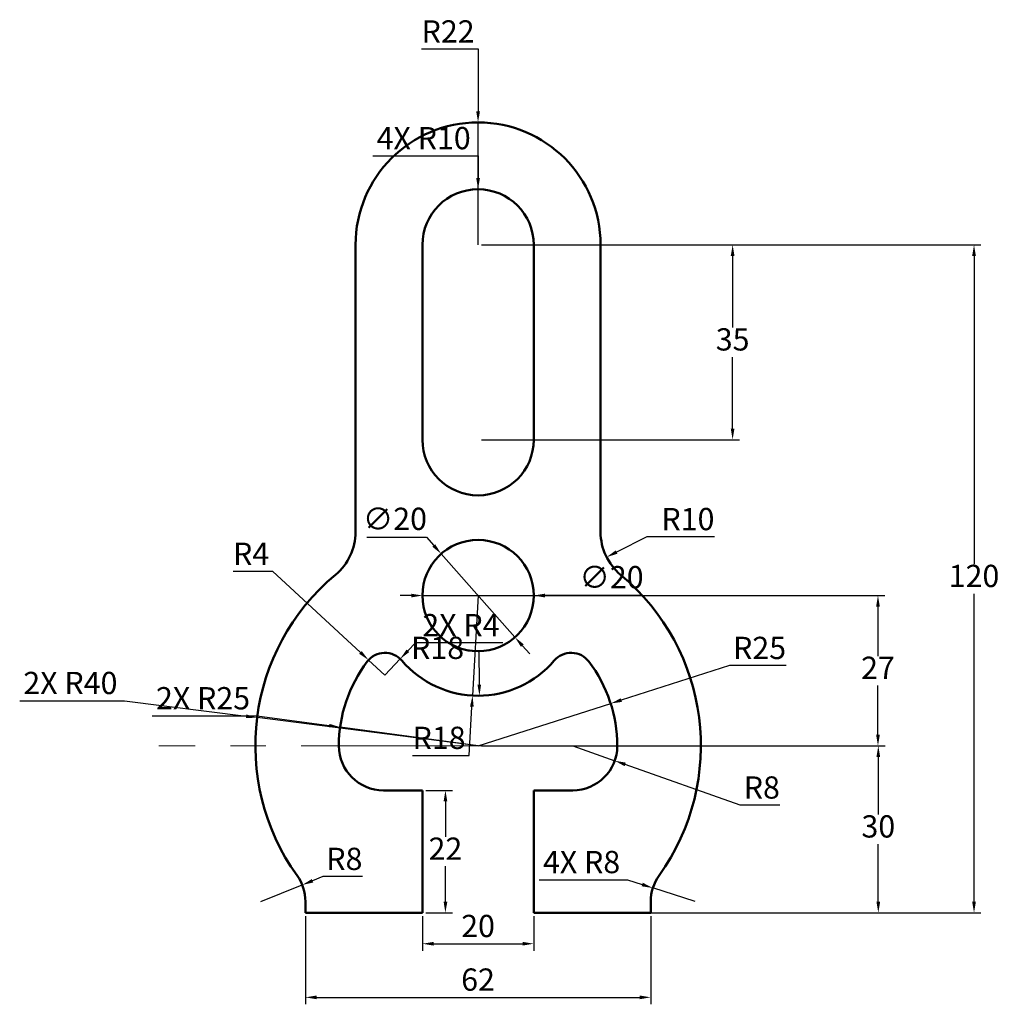
# Model space of a CAD drawing. Units: millimetres. Extents: x 142 to 317, y 52 to 229.
import ezdxf

# ---------------------------------------------------------------- set-up
doc = ezdxf.new("R2010")
doc.units = ezdxf.units.MM
doc.linetypes.add('CENTER', pattern=[50.8, 31.75, -6.35, 6.35, -6.35])
for name, color, linetype, lineweight in [('M-CNTR', 4, 'CENTER', 18), ('M-DIMS', 2, 'Continuous', 25), ('M-OUTL', 7, 'Continuous', 50)]:
    doc.layers.add(name, color=color, linetype=linetype, lineweight=lineweight)
doc.styles.get("Standard").update_dxf_attribs({"font": 'arial.ttf'})
doc.dimstyles.new('ISO-25', dxfattribs={"dimtxt": 4, "dimasz": 2, "dimexe": 1.25, "dimexo": 0.625, "dimtad": 1, "dimtih": 1, "dimtoh": 1, "dimtxsty": 'Standard', "dimcen": 2.5, "dimadec": 0, "dimazin": 0, "dimtfac": 1, "dimtmove": 0, "dimatfit": 3, "dimfxl": 1, "dimarcsym": 0})

# ---------------------------------------------------------------- blocks, each defined once
blk = doc.blocks.new('*D1')
at = {"layer": 'Defpoints', "color": 0, "transparency": 16777216}
for p in [(213.82, 68.93), (233.82, 68.93), (233.82, 63.37)]:
    blk.add_point(p, dxfattribs=at)
at = {"layer": 'M-DIMS', "color": 0, "lineweight": -2, "transparency": 16777216}
for p, q in [((213.82, 68.3), (213.82, 62.12)), ((233.82, 68.3), (233.82, 62.12)), ((215.82, 63.37), (231.82, 63.37))]:
    blk.add_line(p, q, dxfattribs=at)
at = {"layer": 'M-DIMS', "color": 0, "transparency": 16777216}
for points in [[(215.82, 63.7), (215.82, 63.04), (213.82, 63.37)], [(231.82, 63.7), (231.82, 63.04), (233.82, 63.37)]]:
    blk.add_solid(points, dxfattribs=at)
at = {"layer": 'M-DIMS', "color": 0, "transparency": 16777216, "insert": (223.82, 66.04), "char_height": 4, "attachment_point": 5}
blk.add_mtext('20', dxfattribs=at)
blk = doc.blocks.new('*D2')
at = {"layer": 'Defpoints', "color": 0, "transparency": 16777216}
for p in [(192.82, 68.93), (254.82, 68.93), (254.82, 53.74)]:
    blk.add_point(p, dxfattribs=at)
at = {"layer": 'M-DIMS', "color": 0, "lineweight": -2, "transparency": 16777216}
for p, q in [((192.82, 68.3), (192.82, 52.49)), ((254.82, 68.3), (254.82, 52.49)), ((194.82, 53.74), (252.82, 53.74))]:
    blk.add_line(p, q, dxfattribs=at)
at = {"layer": 'M-DIMS', "color": 0, "transparency": 16777216}
for points in [[(194.82, 54.07), (194.82, 53.4), (192.82, 53.74)], [(252.82, 54.07), (252.82, 53.4), (254.82, 53.74)]]:
    blk.add_solid(points, dxfattribs=at)
at = {"layer": 'M-DIMS', "color": 0, "transparency": 16777216, "insert": (223.82, 56.41), "char_height": 4, "attachment_point": 5}
blk.add_mtext('62', dxfattribs=at)
blk = doc.blocks.new('*D3')
at = {"layer": 'Defpoints', "color": 0, "transparency": 16777216}
for p in [(254.82, 98.93), (295.7, 98.93), (254.82, 68.93)]:
    blk.add_point(p, dxfattribs=at)
at = {"layer": 'M-DIMS', "color": 0, "lineweight": -2, "transparency": 16777216}
for p, q in [((255.45, 98.93), (296.95, 98.93)), ((295.7, 96.93), (295.7, 86.59)), ((295.7, 70.93), (295.7, 81.26)), ((255.45, 68.93), (296.95, 68.93))]:
    blk.add_line(p, q, dxfattribs=at)
at = {"layer": 'M-DIMS', "color": 0, "transparency": 16777216}
for points in [[(295.37, 96.93), (296.03, 96.93), (295.7, 98.93)], [(295.37, 70.93), (296.03, 70.93), (295.7, 68.93)]]:
    blk.add_solid(points, dxfattribs=at)
at = {"layer": 'M-DIMS', "color": 0, "transparency": 16777216, "insert": (295.7, 83.93), "char_height": 4, "attachment_point": 5}
blk.add_mtext('30', dxfattribs=at)
blk = doc.blocks.new('*D4')
at = {"layer": 'Defpoints', "color": 0, "transparency": 16777216}
for p in [(223.82, 125.93), (223.82, 98.93), (295.64, 98.93)]:
    blk.add_point(p, dxfattribs=at)
at = {"layer": 'M-DIMS', "color": 0, "lineweight": -2, "transparency": 16777216}
for p, q in [((224.45, 125.93), (296.89, 125.93)), ((295.64, 123.93), (295.64, 115.06)), ((295.64, 100.93), (295.64, 109.79)), ((224.45, 98.93), (296.89, 98.93))]:
    blk.add_line(p, q, dxfattribs=at)
at = {"layer": 'M-DIMS', "color": 0, "transparency": 16777216}
for points in [[(295.31, 123.93), (295.97, 123.93), (295.64, 125.93)], [(295.31, 100.93), (295.97, 100.93), (295.64, 98.93)]]:
    blk.add_solid(points, dxfattribs=at)
at = {"layer": 'M-DIMS', "color": 0, "transparency": 16777216, "insert": (295.64, 112.43), "char_height": 4, "attachment_point": 5}
blk.add_mtext('27', dxfattribs=at)
blk = doc.blocks.new('*D5')
at = {"layer": 'Defpoints', "color": 0, "transparency": 16777216}
for p in [(255.82, 137.34), (246.9, 132.83)]:
    blk.add_point(p, dxfattribs=at)
at = {"layer": 'M-DIMS', "color": 0, "lineweight": -2, "transparency": 16777216}
for p, q in [((254.11, 136.48), (248.69, 133.73)), ((266.28, 136.48), (254.11, 136.48))]:
    blk.add_line(p, q, dxfattribs=at)
at = {"layer": 'M-DIMS', "color": 0, "transparency": 16777216}
blk.add_solid([(248.54, 134.03), (248.84, 133.43), (246.9, 132.83)], dxfattribs=at)
at = {"layer": 'M-DIMS', "color": 0, "transparency": 16777216, "insert": (261.51, 139.15), "char_height": 4, "attachment_point": 5}
blk.add_mtext('R10', dxfattribs=at)
blk = doc.blocks.new('*D6')
at = {"layer": 'Defpoints', "color": 0, "transparency": 16777216}
for p in [(204.16, 114.34), (207.1, 111.63)]:
    blk.add_point(p, dxfattribs=at)
at = {"layer": 'M-DIMS', "color": 0, "lineweight": -2, "transparency": 16777216}
for p, q in [((179.84, 130.29), (186.9, 130.29)), ((186.9, 130.29), (202.69, 115.7)), ((207.1, 111.63), (204.16, 114.34))]:
    blk.add_line(p, q, dxfattribs=at)
at = {"layer": 'M-DIMS', "color": 0, "transparency": 16777216}
blk.add_solid([(202.92, 115.95), (202.47, 115.46), (204.16, 114.34)], dxfattribs=at)
at = {"layer": 'M-DIMS', "color": 0, "transparency": 16777216, "insert": (183.06, 132.92), "char_height": 4, "attachment_point": 5}
blk.add_mtext('R4', dxfattribs=at)
blk = doc.blocks.new('*D7')
at = {"layer": 'Defpoints', "color": 0, "transparency": 16777216}
for p in [(223.82, 125.93), (224.07, 107.93)]:
    blk.add_point(p, dxfattribs=at)
at = {"layer": 'M-DIMS', "color": 0, "lineweight": -2, "transparency": 16777216}
for p, q in [((221.96, 116.01), (223.96, 116.01)), ((223.96, 116.01), (224.04, 109.93))]:
    blk.add_line(p, q, dxfattribs=at)
at = {"layer": 'M-DIMS', "color": 0, "transparency": 16777216}
blk.add_solid([(224.37, 109.93), (223.71, 109.92), (224.07, 107.93)], dxfattribs=at)
at = {"layer": 'M-DIMS', "color": 0, "transparency": 16777216, "insert": (216.55, 116.01), "char_height": 4, "attachment_point": 5}
blk.add_mtext('R18', dxfattribs=at)
blk = doc.blocks.new('*D8')
at = {"layer": 'Defpoints', "color": 0, "transparency": 16777216}
for p in [(213.82, 90.93), (217.96, 90.93), (213.82, 68.93)]:
    blk.add_point(p, dxfattribs=at)
at = {"layer": 'M-DIMS', "color": 0, "lineweight": -2, "transparency": 16777216}
for p, q in [((214.45, 90.93), (219.21, 90.93)), ((217.96, 88.93), (217.96, 82.56)), ((217.96, 70.93), (217.96, 77.29)), ((214.45, 68.93), (219.21, 68.93))]:
    blk.add_line(p, q, dxfattribs=at)
at = {"layer": 'M-DIMS', "color": 0, "transparency": 16777216}
for points in [[(217.63, 88.93), (218.3, 88.93), (217.96, 90.93)], [(217.63, 70.93), (218.3, 70.93), (217.96, 68.93)]]:
    blk.add_solid(points, dxfattribs=at)
at = {"layer": 'M-DIMS', "color": 0, "transparency": 16777216, "insert": (217.96, 79.93), "char_height": 4, "attachment_point": 5}
blk.add_mtext('22', dxfattribs=at)
blk = doc.blocks.new('*D9')
at = {"layer": 'Defpoints', "color": 0, "transparency": 16777216}
for p in [(247.64, 106.53), (223.82, 98.93)]:
    blk.add_point(p, dxfattribs=at)
at = {"layer": 'M-DIMS', "color": 0, "lineweight": -2, "transparency": 16777216}
for p, q in [((268.96, 113.34), (249.54, 107.14)), ((279.17, 113.34), (268.96, 113.34)), ((223.82, 98.93), (247.64, 106.53))]:
    blk.add_line(p, q, dxfattribs=at)
at = {"layer": 'M-DIMS', "color": 0, "transparency": 16777216}
blk.add_solid([(249.44, 107.46), (249.65, 106.82), (247.64, 106.53)], dxfattribs=at)
at = {"layer": 'M-DIMS', "color": 0, "transparency": 16777216, "insert": (274.38, 116), "char_height": 4, "attachment_point": 5}
blk.add_mtext('R25', dxfattribs=at)
blk = doc.blocks.new('*D10')
at = {"layer": 'Defpoints', "color": 0, "transparency": 16777216}
for p in [(240.82, 98.93), (248.36, 96.25)]:
    blk.add_point(p, dxfattribs=at)
at = {"layer": 'M-DIMS', "color": 0, "lineweight": -2, "transparency": 16777216}
for p, q in [((240.82, 98.93), (248.36, 96.25)), ((270.92, 88.25), (250.25, 95.58)), ((278.01, 88.25), (270.92, 88.25))]:
    blk.add_line(p, q, dxfattribs=at)
at = {"layer": 'M-DIMS', "color": 0, "transparency": 16777216}
blk.add_solid([(250.36, 95.9), (250.14, 95.27), (248.36, 96.25)], dxfattribs=at)
at = {"layer": 'M-DIMS', "color": 0, "transparency": 16777216, "insert": (274.78, 90.92), "char_height": 4, "attachment_point": 5}
blk.add_mtext('R8', dxfattribs=at)
blk = doc.blocks.new('*D11')
at = {"layer": 'Defpoints', "color": 0, "transparency": 16777216}
for p in [(192.24, 73.93), (184.82, 70.94)]:
    blk.add_point(p, dxfattribs=at)
at = {"layer": 'M-DIMS', "color": 0, "lineweight": -2, "transparency": 16777216}
for p, q in [((195.95, 75.43), (194.1, 74.68)), ((203.04, 75.43), (195.95, 75.43)), ((184.82, 70.94), (192.24, 73.93))]:
    blk.add_line(p, q, dxfattribs=at)
at = {"layer": 'M-DIMS', "color": 0, "transparency": 16777216}
blk.add_solid([(193.97, 74.99), (194.22, 74.37), (192.24, 73.93)], dxfattribs=at)
at = {"layer": 'M-DIMS', "color": 0, "transparency": 16777216, "insert": (199.81, 78.1), "char_height": 4, "attachment_point": 5}
blk.add_mtext('R8', dxfattribs=at)
blk = doc.blocks.new('*D12')
at = {"layer": 'Defpoints', "color": 0, "transparency": 16777216}
for p in [(223.82, 188.93), (223.82, 153.93), (269.54, 153.93)]:
    blk.add_point(p, dxfattribs=at)
at = {"layer": 'M-DIMS', "color": 0, "lineweight": -2, "transparency": 16777216}
for p, q in [((224.45, 188.93), (270.79, 188.93)), ((269.54, 186.93), (269.54, 174.09)), ((269.54, 155.93), (269.54, 168.76)), ((224.45, 153.93), (270.79, 153.93))]:
    blk.add_line(p, q, dxfattribs=at)
at = {"layer": 'M-DIMS', "color": 0, "transparency": 16777216}
for points in [[(269.2, 186.93), (269.87, 186.93), (269.54, 188.93)], [(269.2, 155.93), (269.87, 155.93), (269.54, 153.93)]]:
    blk.add_solid(points, dxfattribs=at)
at = {"layer": 'M-DIMS', "color": 0, "transparency": 16777216, "insert": (269.54, 171.43), "char_height": 4, "attachment_point": 5}
blk.add_mtext('35', dxfattribs=at)
blk = doc.blocks.new('*D13')
at = {"layer": 'Defpoints', "color": 0, "transparency": 16777216}
for p in [(233.82, 188.93), (312.89, 188.93), (233.82, 68.93)]:
    blk.add_point(p, dxfattribs=at)
at = {"layer": 'M-DIMS', "color": 0, "lineweight": -2, "transparency": 16777216}
for p, q in [((234.45, 188.93), (314.14, 188.93)), ((312.89, 186.93), (312.89, 131.59)), ((312.89, 70.93), (312.89, 126.26)), ((234.45, 68.93), (314.14, 68.93))]:
    blk.add_line(p, q, dxfattribs=at)
at = {"layer": 'M-DIMS', "color": 0, "transparency": 16777216}
for points in [[(312.55, 186.93), (313.22, 186.93), (312.89, 188.93)], [(312.55, 70.93), (313.22, 70.93), (312.89, 68.93)]]:
    blk.add_solid(points, dxfattribs=at)
at = {"layer": 'M-DIMS', "color": 0, "transparency": 16777216, "insert": (312.89, 128.93), "char_height": 4, "attachment_point": 5}
blk.add_mtext('120', dxfattribs=at)
blk = doc.blocks.new('*D14')
at = {"layer": 'Defpoints', "color": 0, "transparency": 16777216}
for p in [(217.2, 133.42), (230.45, 118.43)]:
    blk.add_point(p, dxfattribs=at)
at = {"layer": 'M-DIMS', "color": 0, "lineweight": -2, "transparency": 16777216}
for p, q in [((203.86, 136.41), (214.55, 136.41)), ((214.55, 136.41), (215.87, 134.92)), ((230.45, 118.43), (217.2, 133.42)), ((231.77, 116.94), (233.1, 115.44))]:
    blk.add_line(p, q, dxfattribs=at)
at = {"layer": 'M-DIMS', "color": 0, "transparency": 16777216}
for points in [[(216.12, 135.14), (215.62, 134.69), (217.2, 133.42)], [(232.02, 117.16), (231.52, 116.72), (230.45, 118.43)]]:
    blk.add_solid(points, dxfattribs=at)
at = {"layer": 'M-DIMS', "color": 0, "transparency": 16777216, "insert": (208.89, 139.19), "char_height": 4, "attachment_point": 5}
blk.add_mtext('∅20', dxfattribs=at)
blk = doc.blocks.new('*D15')
at = {"layer": 'Defpoints', "color": 0, "transparency": 16777216}
for p in [(184.15, 103.99), (223.82, 98.93)]:
    blk.add_point(p, dxfattribs=at)
at = {"layer": 'M-DIMS', "color": 0, "lineweight": -2, "transparency": 16777216}
for p, q in [((141.51, 107.03), (160.34, 107.03)), ((160.34, 107.03), (182.16, 104.24)), ((223.82, 98.93), (184.15, 103.99))]:
    blk.add_line(p, q, dxfattribs=at)
at = {"layer": 'M-DIMS', "color": 0, "transparency": 16777216}
blk.add_solid([(182.2, 104.57), (182.12, 103.91), (184.15, 103.99)], dxfattribs=at)
at = {"layer": 'M-DIMS', "color": 0, "transparency": 16777216, "insert": (150.61, 109.7), "char_height": 4, "attachment_point": 5}
blk.add_mtext('2X R40', dxfattribs=at)
blk = doc.blocks.new('*D16')
at = {"layer": 'Defpoints', "color": 0, "transparency": 16777216}
for p in [(223.82, 210.93), (223.82, 188.93)]:
    blk.add_point(p, dxfattribs=at)
at = {"layer": 'M-DIMS', "color": 0, "lineweight": -2, "transparency": 16777216}
for p, q in [((213.68, 224.13), (223.82, 224.13)), ((223.82, 224.13), (223.82, 212.93)), ((223.82, 188.93), (223.82, 210.93))]:
    blk.add_line(p, q, dxfattribs=at)
at = {"layer": 'M-DIMS', "color": 0, "transparency": 16777216}
blk.add_solid([(224.16, 212.93), (223.49, 212.93), (223.82, 210.93)], dxfattribs=at)
at = {"layer": 'M-DIMS', "color": 0, "transparency": 16777216, "insert": (218.44, 226.76), "char_height": 4, "attachment_point": 5}
blk.add_mtext('R22', dxfattribs=at)
blk = doc.blocks.new('*D17')
at = {"layer": 'Defpoints', "color": 0, "transparency": 16777216}
for p in [(223.82, 198.93), (223.82, 188.93)]:
    blk.add_point(p, dxfattribs=at)
at = {"layer": 'M-DIMS', "color": 0, "lineweight": -2, "transparency": 16777216}
for p, q in [((204.9, 204.93), (223.82, 204.93)), ((223.82, 204.93), (223.82, 200.93)), ((223.82, 188.93), (223.82, 198.93))]:
    blk.add_line(p, q, dxfattribs=at)
at = {"layer": 'M-DIMS', "color": 0, "transparency": 16777216}
blk.add_solid([(224.16, 200.93), (223.49, 200.93), (223.82, 198.93)], dxfattribs=at)
at = {"layer": 'M-DIMS', "color": 0, "transparency": 16777216, "insert": (214.05, 207.59), "char_height": 4, "attachment_point": 5}
blk.add_mtext('4X R10', dxfattribs=at)
blk = doc.blocks.new('*D18')
at = {"layer": 'Defpoints', "color": 0, "transparency": 16777216}
for p in [(213.82, 125.93), (233.82, 125.93)]:
    blk.add_point(p, dxfattribs=at)
at = {"layer": 'M-DIMS', "color": 0, "lineweight": -2, "transparency": 16777216}
for p, q in [((211.82, 125.93), (209.82, 125.93)), ((213.82, 125.93), (233.82, 125.93)), ((242.13, 125.93), (235.82, 125.93)), ((252.82, 125.93), (242.13, 125.93))]:
    blk.add_line(p, q, dxfattribs=at)
at = {"layer": 'M-DIMS', "color": 0, "transparency": 16777216}
for points in [[(211.82, 126.26), (211.82, 125.59), (213.82, 125.93)], [(235.82, 126.26), (235.82, 125.59), (233.82, 125.93)]]:
    blk.add_solid(points, dxfattribs=at)
at = {"layer": 'M-DIMS', "color": 0, "transparency": 16777216, "insert": (247.79, 128.71), "char_height": 4, "attachment_point": 5}
blk.add_mtext('∅20', dxfattribs=at)
blk = doc.blocks.new('*D19')
at = {"layer": 'Defpoints', "color": 0, "transparency": 16777216}
for p in [(199.05, 102.28), (223.82, 98.93)]:
    blk.add_point(p, dxfattribs=at)
at = {"layer": 'M-DIMS', "color": 0, "lineweight": -2, "transparency": 16777216}
for p, q in [((165.31, 104.29), (184.18, 104.29)), ((184.18, 104.29), (197.07, 102.55)), ((223.82, 98.93), (199.05, 102.28))]:
    blk.add_line(p, q, dxfattribs=at)
at = {"layer": 'M-DIMS', "color": 0, "transparency": 16777216}
blk.add_solid([(197.11, 102.88), (197.02, 102.22), (199.05, 102.28)], dxfattribs=at)
at = {"layer": 'M-DIMS', "color": 0, "transparency": 16777216, "insert": (174.43, 106.96), "char_height": 4, "attachment_point": 5}
blk.add_mtext('2X R25', dxfattribs=at)
blk = doc.blocks.new('*D20')
at = {"layer": 'Defpoints', "color": 0, "transparency": 16777216}
for p in [(223.82, 125.93), (222.82, 107.95)]:
    blk.add_point(p, dxfattribs=at)
at = {"layer": 'M-DIMS', "color": 0, "lineweight": -2, "transparency": 16777216}
for p, q in [((223.82, 125.93), (222.82, 107.95)), ((222.22, 97.17), (222.71, 105.96)), ((212.03, 97.17), (222.22, 97.17))]:
    blk.add_line(p, q, dxfattribs=at)
at = {"layer": 'M-DIMS', "color": 0, "transparency": 16777216}
blk.add_solid([(222.38, 105.98), (223.04, 105.94), (222.82, 107.95)], dxfattribs=at)
at = {"layer": 'M-DIMS', "color": 0, "transparency": 16777216, "insert": (216.82, 99.84), "char_height": 4, "attachment_point": 5}
blk.add_mtext('R18', dxfattribs=at)
blk = doc.blocks.new('*D21')
at = {"layer": 'Defpoints', "color": 0, "transparency": 16777216}
for p in [(209.84, 114.54), (207.1, 111.63)]:
    blk.add_point(p, dxfattribs=at)
at = {"layer": 'M-DIMS', "color": 0, "lineweight": -2, "transparency": 16777216}
for p, q in [((212.58, 117.46), (211.21, 116)), ((228.3, 117.46), (212.58, 117.46)), ((207.1, 111.63), (209.84, 114.54))]:
    blk.add_line(p, q, dxfattribs=at)
at = {"layer": 'M-DIMS', "color": 0, "transparency": 16777216}
blk.add_solid([(210.97, 116.23), (211.45, 115.77), (209.84, 114.54)], dxfattribs=at)
at = {"layer": 'M-DIMS', "color": 0, "transparency": 16777216, "insert": (220.75, 120.09), "char_height": 4, "attachment_point": 5}
blk.add_mtext('2X R4', dxfattribs=at)
blk = doc.blocks.new('*D22')
at = {"layer": 'Defpoints', "color": 0, "transparency": 16777216}
for p in [(255.21, 73.39), (262.82, 70.94)]:
    blk.add_point(p, dxfattribs=at)
at = {"layer": 'M-DIMS', "color": 0, "lineweight": -2, "transparency": 16777216}
for p, q in [((234.8, 74.86), (250.64, 74.86)), ((250.64, 74.86), (253.3, 74.01)), ((262.82, 70.94), (255.21, 73.39))]:
    blk.add_line(p, q, dxfattribs=at)
at = {"layer": 'M-DIMS', "color": 0, "transparency": 16777216}
blk.add_solid([(253.41, 74.32), (253.2, 73.69), (255.21, 73.39)], dxfattribs=at)
at = {"layer": 'M-DIMS', "color": 0, "transparency": 16777216, "insert": (242.41, 77.53), "char_height": 4, "attachment_point": 5}
blk.add_mtext('4X R8', dxfattribs=at)

msp = doc.modelspace()

# ---------------------------------------------------------------- linework, layer by layer
at = {"layer": 'M-CNTR'}
for q in [(166.522, 98.926), (274.536, 98.926)]:
    msp.add_line((223.823, 98.926), q, dxfattribs=at)
at = {"layer": 'M-OUTL'}
for p, q in [((201.823, 188.926), (201.823, 153.926)), ((213.823, 188.926), (213.823, 173.522)), ((233.823, 188.926), (233.823, 173.522)), ((245.823, 188.926), (245.823, 153.926)), ((213.823, 173.522), (213.823, 153.926)), ((233.823, 153.926), (233.823, 173.522)), ((201.823, 153.926), (201.823, 137.345)), ((245.823, 153.926), (245.823, 137.345)), ((213.823, 90.926), (206.823, 90.926)), ((213.823, 68.926), (213.823, 90.926)), ((233.823, 68.926), (233.823, 90.926)), ((233.823, 90.926), (240.823, 90.926)), ((192.823, 68.926), (192.823, 70.944)), ((254.823, 68.926), (254.823, 70.944)), ((192.823, 68.926), (213.823, 68.926)), ((233.823, 68.926), (254.823, 68.926))]:
    msp.add_line(p, q, dxfattribs=at)
msp.add_circle((223.823, 125.926), 10, dxfattribs=at)
for centre, radius, start, end in [((223.823, 188.926), 22, 0, 180), ((223.823, 188.926), 10, 0, 180), ((223.823, 153.926), 10, 180, 0), ((191.823, 137.345), 10, 309.79182, 0), ((255.823, 137.345), 10, 180, 230.20818), ((223.823, 98.926), 40, 129.79182, 215.65909), ((223.823, 98.926), 40, 324.34091, 50.20818), ((207.101, 111.63), 4, 40.52891, 142.7756), ((240.545, 111.63), 4, 37.2244, 139.47109), ((223.823, 98.926), 25, 142.7756, 180), ((223.823, 125.926), 18, 220.52891, 319.47109), ((223.823, 98.926), 25, 0, 37.2244), ((206.823, 98.926), 8, 180, 270), ((240.823, 98.926), 8, 270, 0), ((184.823, 70.944), 8, 0, 35.65909), ((262.823, 70.944), 8, 144.34091, 180)]:
    msp.add_arc(centre, radius, start, end, dxfattribs=at)

# ---------------------------------------------------------------- dimensions: what is measured, and where the dimension line sits
at = {"layer": 'M-DIMS'}
for center, mpoint, override, picture, middle in [((223.823, 188.926), (223.823, 210.926), {"dimdec": 0, "dimlfac": 1, "dimrnd": 0, "dimzin": 0, "dimdsep": 46, "dimlunit": 2}, '*D16', (218.439, 224.126)), ((255.823, 137.345), (246.902, 132.828), {"dimclrd": 0, "dimclre": 0, "dimclrt": 0}, '*D5', (261.511, 136.48)), ((207.101, 111.63), (204.163, 114.344), {"dimclrd": 0, "dimclre": 0, "dimclrt": 0}, '*D6', (183.06, 130.292)), ((223.823, 125.926), (224.068, 107.928), {"dimclrd": 0, "dimclre": 0, "dimclrt": 0}, '*D7', (216.55, 116.012)), ((223.823, 125.926), (222.823, 107.954), {"dimdec": 0, "dimlfac": 1, "dimrnd": 0, "dimzin": 0, "dimdsep": 46, "dimlunit": 2}, '*D20', (216.815, 97.171)), ((223.823, 98.926), (247.639, 106.529), {"dimclrd": 0, "dimclre": 0, "dimclrt": 0}, '*D9', (274.381, 113.337)), ((240.823, 98.926), (248.363, 96.252), {"dimclrd": 0, "dimclre": 0, "dimclrt": 0}, '*D10', (274.779, 88.252))]:
    dim = msp.add_radius_dim(center=center, mpoint=mpoint, dimstyle='ISO-25', override=override, dxfattribs=at)
    dim.commit()
    dim.dimension.update_dxf_attribs({"geometry": picture, "text_midpoint": middle, "dimtype": 164})
for center, mpoint, text, picture, middle in [((223.823, 188.926), (223.823, 198.926), '4X <>', '*D17', (214.048, 204.926)), ((223.823, 98.926), (184.145, 103.991), '2X <>', '*D15', (160.338, 107.03)), ((223.823, 98.926), (199.049, 102.28), '2X <>', '*D19', (184.185, 104.293)), ((262.823, 70.944), (255.207, 73.393), '4X <>', '*D22', (242.406, 74.862))]:
    dim = msp.add_radius_dim(center=center, mpoint=mpoint, text=text, dimstyle='ISO-25', override={"dimdec": 0, "dimlfac": 1, "dimrnd": 0, "dimzin": 0, "dimdsep": 46, "dimlunit": 2}, dxfattribs=at)
    dim.commit()
    dim.dimension.update_dxf_attribs({"geometry": picture, "text_midpoint": middle, "dimtype": 164})
for base, p1, p2, picture, middle in [((269.537, 153.926), (223.823, 188.926), (223.823, 153.926), '*D12', (269.537, 171.426)), ((312.886, 188.926), (233.823, 68.926), (233.823, 188.926), '*D13', (312.886, 128.926)), ((295.641, 98.926), (223.823, 125.926), (223.823, 98.926), '*D4', (295.641, 112.426)), ((295.701, 98.926), (254.823, 68.926), (254.823, 98.926), '*D3', (295.701, 83.926)), ((217.963, 90.926), (213.823, 68.926), (213.823, 90.926), '*D8', (217.963, 79.926))]:
    dim = msp.add_linear_dim(base=base, p1=p1, p2=p2, angle=90, dimstyle='ISO-25', override={"dimclrd": 0, "dimclre": 0, "dimclrt": 0}, dxfattribs=at)
    dim.commit()
    dim.dimension.update_dxf_attribs({"geometry": picture, "text_midpoint": middle})
for p1, p2, override, picture, middle in [((230.447, 118.435), (217.199, 133.417), {"dimclrd": 0, "dimclre": 0, "dimclrt": 0}, '*D14', (208.89, 136.414)), ((213.823, 125.926), (233.823, 125.926), {"dimdec": 0, "dimlfac": 1, "dimrnd": 0, "dimzin": 0, "dimdsep": 46, "dimlunit": 2}, '*D18', (242.131, 125.926))]:
    dim = msp.add_diameter_dim_2p(p1=p1, p2=p2, dimstyle='ISO-25', override=override, dxfattribs=at)
    dim.commit()
    dim.dimension.update_dxf_attribs({"geometry": picture, "text_midpoint": middle, "dimtype": 163})
dim = msp.add_radius_dim(center=(207.101, 111.63), mpoint=(209.841, 114.544), text='2X <>', dimstyle='ISO-25', override={"dimdec": 0, "dimlfac": 1, "dimrnd": 0, "dimzin": 0, "dimdsep": 46, "dimlunit": 2}, dxfattribs=at)
dim.commit()
dim.dimension.update_dxf_attribs({"geometry": '*D21', "text_midpoint": (220.755, 120.093)})
dim = msp.add_radius_dim(center=(184.823, 70.944), mpoint=(192.243, 73.935), dimstyle='ISO-25', override={"dimclrd": 0, "dimclre": 0, "dimclrt": 0}, dxfattribs=at)
dim.commit()
dim.dimension.update_dxf_attribs({"geometry": '*D11', "text_midpoint": (199.807, 78.097)})
for base, p1, p2, picture, middle in [((254.823, 53.738), (192.823, 68.926), (254.823, 68.926), '*D2', (223.823, 56.405)), ((233.823, 63.369), (213.823, 68.926), (233.823, 68.926), '*D1', (223.823, 66.036))]:
    dim = msp.add_linear_dim(base=base, p1=p1, p2=p2, dimstyle='ISO-25', override={"dimclrd": 0, "dimclre": 0, "dimclrt": 0}, dxfattribs=at)
    dim.commit()
    dim.dimension.update_dxf_attribs({"geometry": picture, "text_midpoint": middle})

doc.saveas('drawing.dxf')
